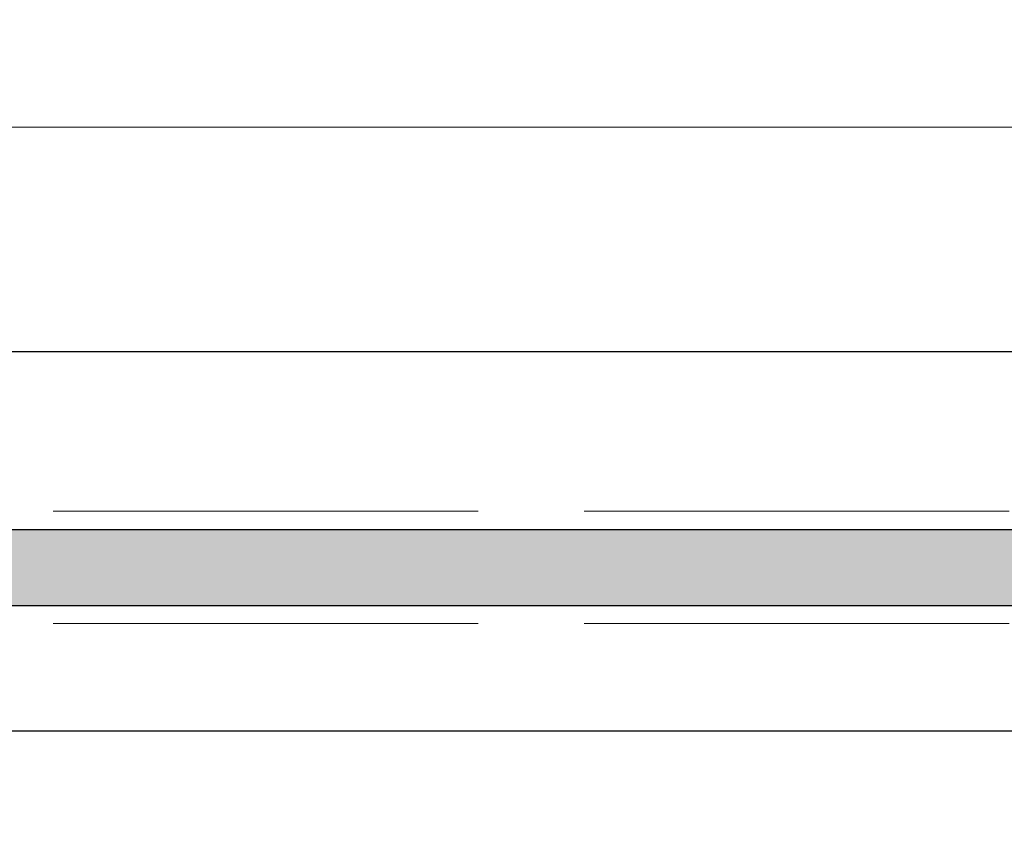
# Model space of a CAD drawing. Units: millimetres. Extents: x 595116 to 630915, y 909473 to 920225.
# Tile 32 of 134: x 629654 to 629682, y 919141 to 919164. Entities that reach past the tile are written whole.
import ezdxf

# ---------------------------------------------------------------- set-up
doc = ezdxf.new("R2010")
doc.units = ezdxf.units.MM
doc.linetypes.add('ACAD_ISO02W100', pattern=[15, 12, -3])
for name, color, linetype, lineweight in [('C-PROP', 7, 'Continuous', 25), ('C-PROP-REF', 240, 'ACAD_ISO02W100', 13), ('Dimension', 3, 'Continuous', 18), ('L-PLNT', 85, 'Continuous', 13)]:
    doc.layers.add(name, color=color, linetype=linetype, lineweight=lineweight)
doc.styles.get("Standard").update_dxf_attribs({"font": 'arial.ttf'})
doc.dimstyles.new('ISO-25', dxfattribs={"dimtxt": 9, "dimasz": 6, "dimexe": 1.25, "dimexo": 0.625, "dimtad": 1, "dimlunit": 4, "dimtxsty": 'Standard', "dimcen": 2.5, "dimadec": 0, "dimazin": 0, "dimtfac": 1, "dimtmove": 0, "dimatfit": 3, "dimfxl": 1, "dimarcsym": 0})

# ---------------------------------------------------------------- blocks, each defined once
blk = doc.blocks.new('*D216')
at = {"layer": 'Defpoints', "color": 0, "transparency": 16777216}
for p in [(629505.041, 919411.828), (629743.541, 919411.928), (629743.541, 918832.378)]:
    blk.add_point(p, dxfattribs=at)
at = {"layer": 'Dimension', "color": 0, "lineweight": -2, "transparency": 16777216}
for p, q in [((629505.041, 919411.203), (629505.041, 918831.128)), ((629743.541, 919411.303), (629743.541, 918831.128)), ((629511.041, 918832.378), (629737.541, 918832.378))]:
    blk.add_line(p, q, dxfattribs=at)
at = {"layer": 'Dimension', "color": 0, "transparency": 16777216}
for points in [[(629511.041, 918833.378), (629511.041, 918831.378), (629505.041, 918832.378)], [(629737.541, 918833.378), (629737.541, 918831.378), (629743.541, 918832.378)]]:
    blk.add_solid(points, dxfattribs=at)
at = {"layer": 'Dimension', "color": 0, "transparency": 16777216, "insert": (629624.291, 918837.656), "char_height": 9, "attachment_point": 5}
blk.add_mtext('19\'-10 1/2"', dxfattribs=at)

msp = doc.modelspace()

# ---------------------------------------------------------------- hatches: boundary and pattern name
at = {"layer": 'C-PROP'}
h = msp.add_hatch(color=256, dxfattribs=at)
h.dxf.hatch_style = 1
h.paths.add_polyline_path([(629809.541, 919149.555), (629625.041, 919149.555), (629625.041, 919147.413), (629809.541, 919147.413)])

# ---------------------------------------------------------------- linework, layer by layer
for p, q in [((629625.041, 919149.555), (629809.541, 919149.555)), ((629625.041, 919147.413), (629809.541, 919147.413))]:
    msp.add_line(p, q, dxfattribs=at)
msp.add_lwpolyline([(629809.541, 919143.864), (629625.041, 919143.864), (629625.041, 919154.587), (629809.541, 919154.587)], close=True, dxfattribs=at)
at = {"layer": 'C-PROP-REF'}
for p, q in [((629625.041, 919150.076), (629809.541, 919150.076)), ((629625.041, 919146.905), (629809.541, 919146.905))]:
    msp.add_line(p, q, dxfattribs=at)
at = {"layer": 'L-PLNT'}
msp.add_line((629511.274, 919160.917), (629824.951, 919160.917), dxfattribs=at)

# ---------------------------------------------------------------- dimensions: what is measured, and where the dimension line sits
at = {"layer": 'Dimension'}
dim = msp.add_linear_dim(base=(629743.541, 918832.378), p1=(629505.041, 919411.828), p2=(629743.541, 919411.928), dimstyle='ISO-25', override={"dimdec": 1, "dimlfac": 1, "dimrnd": 0, "dimzin": 1, "dimdsep": 46, "dimlunit": 4, "dimfrac": 2}, dxfattribs=at)
dim.commit()
dim.dimension.update_dxf_attribs({"geometry": '*D216', "text_midpoint": (629624.291, 918837.656)})

doc.saveas('drawing.dxf')
